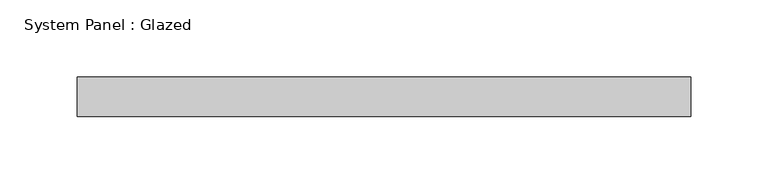
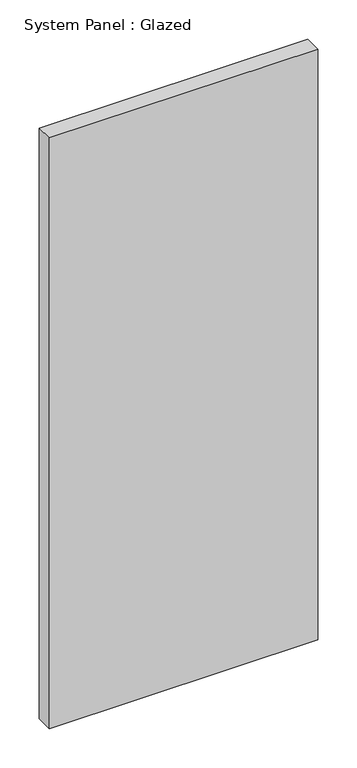
"""IFC4 building model written with IfcOpenShell, lengths in millimetres: plate geometry, System Panel : Glazed."""

from ifc_helpers import new_model, si_unit, origin, origin_with_axes, place, context, project, spatial, polyline, outline, extrude, source, transform, mapped, element, save


def system_panel_glazed_323f7165(model_context):
    return source(origin(), model_context, "Body", "SweptSolid", [
        extrude(outline(polyline([(197.9083333, 19.05), (-197.9083333, 19.05), (-197.9083333, 44.45), (197.9083333, 44.45), (197.9083333, 19.05)])), origin_with_axes(), (0.0, 0.0, 1.0), 920.75),
    ])


if __name__ == "__main__":
    model = new_model("IFC4")
    model_context = context("Model", 3, world=origin())
    ifc_project = project(units=[si_unit("LENGTHUNIT", "METRE", prefix="MILLI")], contexts=[model_context])
    site = spatial("IfcSite", under=ifc_project)
    building = spatial("IfcBuilding", under=site)
    placement = place(None, origin())
    system_panel_glazed_shape = system_panel_glazed_323f7165(model_context)
    element("IfcPlate", 1, ObjectType="System Panel : Glazed", at=placement, inside=building, context=model_context, shape_type="MappedRepresentation", body=[
        mapped(system_panel_glazed_shape, transform((0.0, 0.0, 0.0), x_axis=(1.0, 0.0, 0.0), y_axis=(0.0, 1.0, 0.0), z_axis=(0.0, 0.0, 1.0))),
    ])
    save(model, "model.ifc")

# Revit data of these elements
# Type "System Panel : Glazed"
#   Construction Type Id = "GSP4R"
#   Analytic Construction = "1/8 in Pilkington single glazing"
#   Visual Light Transmittance = 0.9
#   Solar Heat Gain Coefficient = 0.86
#   Heat Transfer Coefficient (U) = 1.18115 BTU/(h·ft²·°F)
#   Define Thermal Properties by = 1
# Element 1 (IfcPlate, "System Panel : Glazed")
#   Materials on its faces: "Glass"
# Materials
#   "Glass": class "Glass", colour RGB 0 128 192, transparency 0.75, Description = "Soda Lime Glass", Cost = 0
